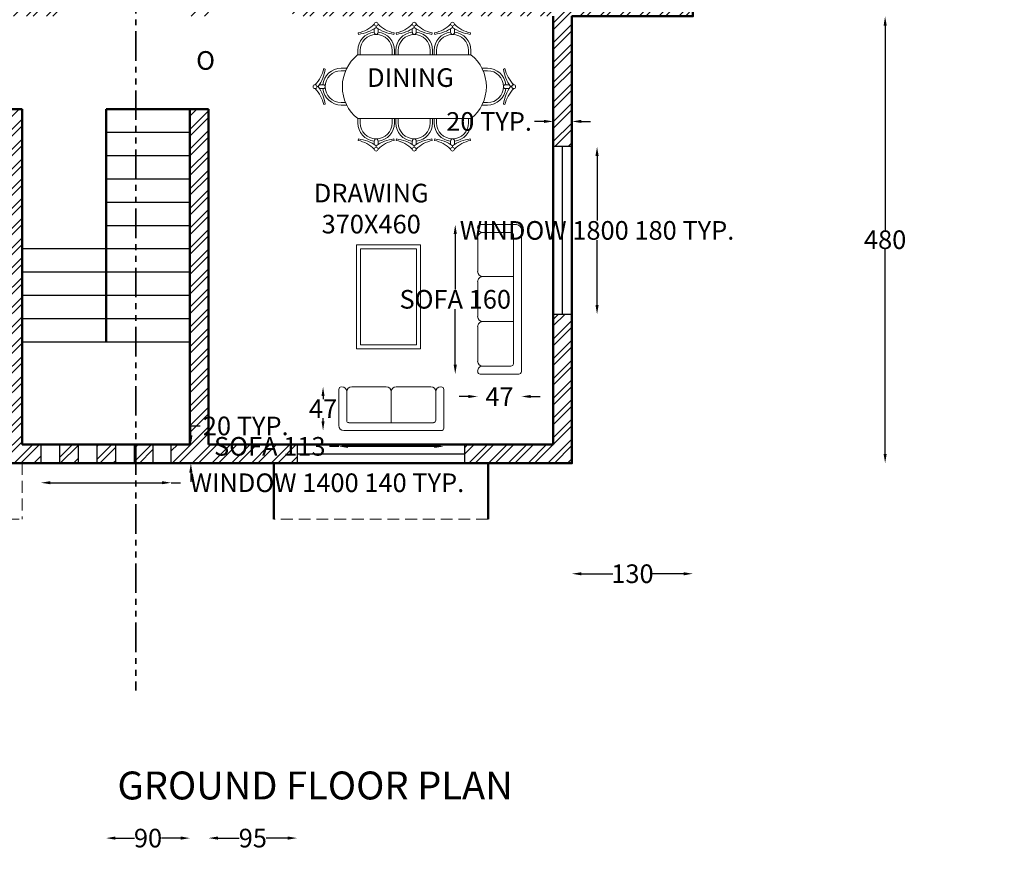
# Model space of a CAD drawing. Units: centimetres. Extents: x 10444 to 13814, y 8288 to 11191.
# Tile 3 of 9: x 11072 to 12129, y 9505 to 10397. Entities that reach past the tile are written whole.
import ezdxf

# ---------------------------------------------------------------- set-up
doc = ezdxf.new("R2010")
doc.units = ezdxf.units.CM
doc.header["$MEASUREMENT"] = 0
doc.linetypes.add('DASHED', pattern=[19.05, 12.7, -6.35])
doc.linetypes.add('PHANTOM', pattern=[63.5, 31.75, -6.35, 6.35, -6.35, 6.35, -6.35])
for name, color, linetype, lineweight in [('A-ANNO-DIMS', 2, 'Continuous', 18), ('A-ANNO-SYMB-SECT', 1, 'PHANTOM', 35), ('A-ANNO-TEXT', 7, 'Continuous', 25), ('A-AREA-IDEN', 3, 'Continuous', 25), ('A-FLOR-STRS', 3, 'Continuous', 25), ('A-FURN', 8, 'Continuous', 18), ('A-GLAZ', 4, 'Continuous', 25), ('A-ROOF-OVHD', 6, 'DASHED', 18), ('A-WALL', 7, 'Continuous', 50), ('A-WALL-PATT', 8, 'Continuous', 13)]:
    doc.layers.add(name, color=color, linetype=linetype, lineweight=lineweight)
doc.styles.get("Standard").update_dxf_attribs({"font": 'arial.ttf'})
doc.dimstyles.get("Standard").update_dxf_attribs({"dimtxt": 20, "dimasz": 10, "dimexe": 0.18, "dimexo": 0.0625, "dimgap": 0.09, "dimtad": 0, "dimtih": 1, "dimtoh": 1, "dimdec": 0, "dimzin": 0, "dimdsep": 46, "dimtxsty": 'Standard', "dimcen": 0.09, "dimse1": 1, "dimse2": 1, "dimadec": 0, "dimazin": 0, "dimtfac": 1, "dimtdec": 0, "dimtofl": 0, "dimtmove": 0, "dimatfit": 3, "dimfxl": 1, "dimtolj": 1, "dimtzin": 0, "dimarcsym": 0})

# ---------------------------------------------------------------- blocks, each defined once
blk = doc.blocks.new('sofa-25')
at = {"color": 0, "linetype": 'ByBlock'}
for p, q in [((-0.03, 0.03), (-0.03, 0.49)), ((0.535, 0.52), (0.124, 0.52)), ((1.07, 0.52), (0.653, 0.52)), ((1.594, 0.52), (1.188, 0.52)), ((1.747, 0.059), (1.747, 0.49)), ((0.065, 0.124), (0.065, 0.461)), ((0.594, 0.094), (0.594, 0.461)), ((1.129, 0.094), (1.129, 0.461)), ((1.653, 0.118), (1.653, 0.461)), ((0, 0), (1.688, 0)), ((0.094, 0.094), (1.629, 0.094))]:
    blk.add_line(p, q, dxfattribs=at)
for centre, radius, start, end in [((0, 0.49), 0.0295, 90, 180), ((0.006, 0.461), 0.0591, 0, 90), ((0.124, 0.461), 0.0591, 90, 180), ((0.535, 0.461), 0.0591, 0, 90), ((0.653, 0.461), 0.0591, 90, 180), ((1.07, 0.461), 0.0591, 0, 90), ((1.188, 0.461), 0.0591, 90, 180), ((1.594, 0.461), 0.0591, 0, 90), ((1.712, 0.461), 0.0591, 90, 180), ((1.718, 0.49), 0.0295, 0, 90), ((0.094, 0.124), 0.0295, 180, 270), ((1.629, 0.118), 0.0236, 270, 0), ((0, 0.03), 0.0295, 180, 270), ((1.688, 0.059), 0.0591, 270, 0)]:
    blk.add_arc(centre, radius, start, end, dxfattribs=at)
blk = doc.blocks.new('sofa-26')
at = {"color": 0, "linetype": 'ByBlock'}
for p, q in [((-0.03, 0.03), (-0.03, 0.49)), ((0.535, 0.52), (0.124, 0.52)), ((1.064, 0.52), (0.653, 0.52)), ((1.218, 0.059), (1.218, 0.49)), ((0.065, 0.124), (0.065, 0.461)), ((0.594, 0.094), (0.594, 0.461)), ((1.123, 0.118), (1.123, 0.461)), ((0, 0), (1.159, 0)), ((0.094, 0.094), (1.1, 0.094))]:
    blk.add_line(p, q, dxfattribs=at)
for centre, radius, start, end in [((0, 0.49), 0.0295, 90, 180), ((0.006, 0.461), 0.0591, 0, 90), ((0.124, 0.461), 0.0591, 90, 180), ((0.535, 0.461), 0.0591, 0, 90), ((0.653, 0.461), 0.0591, 90, 180), ((1.064, 0.461), 0.0591, 0, 90), ((1.182, 0.461), 0.0591, 90, 180), ((1.188, 0.49), 0.0295, 0, 90), ((0.094, 0.124), 0.0295, 180, 270), ((1.1, 0.118), 0.0236, 270, 0), ((0, 0.03), 0.0295, 180, 270), ((1.159, 0.059), 0.0591, 270, 0)]:
    blk.add_arc(centre, radius, start, end, dxfattribs=at)
blk = doc.blocks.new('*D9')
at = {"layer": 'A-ANNO-DIMS', "color": 0, "lineweight": -2, "transparency": 16777216}
for p, q in [((12001, 10390.6), (12001, 10170.9)), ((12001, 9930.6), (12001, 10150.3))]:
    blk.add_line(p, q, dxfattribs=at)
at = {"layer": 'A-ANNO-DIMS', "color": 0, "transparency": 16777216}
for points in [[(11999.4, 10390.6), (12002.7, 10390.6), (12001, 10400.6)], [(11999.4, 9930.6), (12002.7, 9930.6), (12001, 9920.6)]]:
    blk.add_solid(points, dxfattribs=at)
at = {"layer": 'Defpoints', "color": 0, "transparency": 16777216}
for p in [(11664.8, 10400.6), (11664.8, 9920.6), (12001, 9920.6)]:
    blk.add_point(p, dxfattribs=at)
at = {"layer": 'A-ANNO-DIMS', "color": 0, "transparency": 16777216, "insert": (12001, 10160.6), "char_height": 20, "attachment_point": 5}
blk.add_mtext('\\A1;480', dxfattribs=at)
blk = doc.blocks.new('*D14')
at = {"layer": 'A-ANNO-DIMS', "color": 0, "lineweight": -2, "transparency": 16777216}
for p, q in [((11674.8, 9801.9), (11708.6, 9801.9)), ((11784.8, 9801.9), (11751, 9801.9))]:
    blk.add_line(p, q, dxfattribs=at)
at = {"layer": 'A-ANNO-DIMS', "color": 0, "transparency": 16777216}
for points in [[(11674.8, 9803.5), (11674.8, 9800.2), (11664.8, 9801.9)], [(11784.8, 9803.5), (11784.8, 9800.2), (11794.8, 9801.9)]]:
    blk.add_solid(points, dxfattribs=at)
at = {"layer": 'Defpoints', "color": 0, "transparency": 16777216}
for p in [(11664.8, 10400.6), (11794.8, 10400.6), (11664.8, 9801.9)]:
    blk.add_point(p, dxfattribs=at)
at = {"layer": 'A-ANNO-DIMS', "color": 0, "transparency": 16777216, "insert": (11729.8, 9801.9), "char_height": 20, "attachment_point": 5}
blk.add_mtext('\\A1;130', dxfattribs=at)
blk = doc.blocks.new('f')
for p, q in [((11304.7, 9881.5), (11164.7, 9881.5)), ((11164.7, 9881.5), (11164.7, 9861.5)), ((11184.7, 9881.5), (11184.7, 9861.5)), ((11204.7, 9881.5), (11204.7, 9861.5)), ((11224.7, 9881.5), (11224.7, 9861.5)), ((11244.7, 9881.5), (11244.7, 9861.5)), ((11264.7, 9881.5), (11264.7, 9861.5)), ((11284.7, 9881.5), (11284.7, 9861.5)), ((11304.7, 9861.5), (11304.7, 9881.5)), ((11164.7, 9861.5), (11304.7, 9861.5))]:
    blk.add_line(p, q)
blk = doc.blocks.new('WIN-1800')
blk.add_line((0, 10), (180, 10))
blk.add_lwpolyline([(0, 0), (180, 0), (180, 20), (0, 20)], close=True)
blk = doc.blocks.new('*D31')
at = {"layer": 'A-ANNO-DIMS', "color": 0, "lineweight": -2, "transparency": 16777216}
for p, q in [((11691.8, 10250.6), (11691.8, 10181.1)), ((11691.8, 10090.6), (11691.8, 10160.2))]:
    blk.add_line(p, q, dxfattribs=at)
at = {"layer": 'A-ANNO-DIMS', "color": 0, "transparency": 16777216}
for points in [[(11690.1, 10250.6), (11693.5, 10250.6), (11691.8, 10260.6)], [(11690.1, 10090.6), (11693.5, 10090.6), (11691.8, 10080.6)]]:
    blk.add_solid(points, dxfattribs=at)
at = {"layer": 'Defpoints', "color": 0, "transparency": 16777216}
for p in [(11664.8, 10260.6), (11691.8, 10260.6), (11664.8, 10080.6)]:
    blk.add_point(p, dxfattribs=at)
at = {"layer": 'A-ANNO-DIMS', "color": 0, "transparency": 16777216, "insert": (11691.8, 10170.6), "char_height": 20, "attachment_point": 5}
blk.add_mtext('\\A1;WINDOW 1800 180 TYP.', dxfattribs=at)
blk = doc.blocks.new('*D32')
at = {"layer": 'A-ANNO-DIMS', "color": 0, "lineweight": -2, "transparency": 16777216}
for p, q in [((11634.8, 10287.6), (11624.8, 10287.6)), ((11674.8, 10287.6), (11684.8, 10287.6))]:
    blk.add_line(p, q, dxfattribs=at)
at = {"layer": 'A-ANNO-DIMS', "color": 0, "transparency": 16777216}
for points in [[(11634.8, 10289.3), (11634.8, 10286), (11644.8, 10287.6)], [(11674.8, 10289.3), (11674.8, 10286), (11664.8, 10287.6)]]:
    blk.add_solid(points, dxfattribs=at)
at = {"layer": 'Defpoints', "color": 0, "transparency": 16777216}
for p in [(11644.8, 10287.6), (11644.8, 10260.6), (11664.8, 10260.6)]:
    blk.add_point(p, dxfattribs=at)
at = {"layer": 'A-ANNO-DIMS', "color": 0, "transparency": 16777216, "insert": (11575.9, 10287.6), "char_height": 20, "attachment_point": 5}
blk.add_mtext('\\A1;20 TYP.', dxfattribs=at)
blk = doc.blocks.new('*D35')
at = {"layer": 'A-ANNO-DIMS', "color": 0, "lineweight": -2, "transparency": 16777216}
for p, q in [((11104.8, 9899.6), (11224.8, 9899.6)), ((11234.8, 9899.6), (11244.8, 9899.6))]:
    blk.add_line(p, q, dxfattribs=at)
at = {"layer": 'A-ANNO-DIMS', "color": 0, "transparency": 16777216}
for points in [[(11104.8, 9901.3), (11104.8, 9898), (11094.8, 9899.6)], [(11224.8, 9901.3), (11224.8, 9898), (11234.8, 9899.6)]]:
    blk.add_solid(points, dxfattribs=at)
at = {"layer": 'Defpoints', "color": 0, "transparency": 16777216}
for p in [(11094.8, 9920.6), (11234.8, 9920.6), (11234.8, 9899.6)]:
    blk.add_point(p, dxfattribs=at)
at = {"layer": 'A-ANNO-DIMS', "color": 0, "transparency": 16777216, "insert": (11401.9, 9899.6), "char_height": 20, "attachment_point": 5}
blk.add_mtext('\\A1;WINDOW 1400 140 TYP.', dxfattribs=at)
blk = doc.blocks.new('*D36')
at = {"layer": 'A-ANNO-DIMS', "color": 0, "lineweight": -2, "transparency": 16777216}
for p, q in [((11255.8, 9950.6), (11255.8, 9960.6)), ((11255.8, 9960.6), (11265.8, 9960.6)), ((11255.8, 9910.6), (11255.8, 9900.6))]:
    blk.add_line(p, q, dxfattribs=at)
at = {"layer": 'A-ANNO-DIMS', "color": 0, "transparency": 16777216}
for points in [[(11254.1, 9950.6), (11257.5, 9950.6), (11255.8, 9940.6)], [(11254.1, 9910.6), (11257.5, 9910.6), (11255.8, 9920.6)]]:
    blk.add_solid(points, dxfattribs=at)
at = {"layer": 'Defpoints', "color": 0, "transparency": 16777216}
for p in [(11234.8, 9940.6), (11255.8, 9940.6), (11234.8, 9920.6)]:
    blk.add_point(p, dxfattribs=at)
at = {"layer": 'A-ANNO-DIMS', "color": 0, "transparency": 16777216, "insert": (11314.7, 9960.6), "char_height": 20, "attachment_point": 5}
blk.add_mtext('\\A1;20 TYP.', dxfattribs=at)
blk = doc.blocks.new('*D45')
at = {"layer": 'A-ANNO-DIMS', "color": 0, "lineweight": -2, "transparency": 16777216}
for p, q in [((11539.6, 10166.8), (11539.6, 10107)), ((11539.6, 10026.3), (11539.6, 10086.1))]:
    blk.add_line(p, q, dxfattribs=at)
at = {"layer": 'A-ANNO-DIMS', "color": 0, "transparency": 16777216}
for points in [[(11537.9, 10166.8), (11541.3, 10166.8), (11539.6, 10176.8)], [(11537.9, 10026.3), (11541.3, 10026.3), (11539.6, 10016.3)]]:
    blk.add_solid(points, dxfattribs=at)
at = {"layer": 'Defpoints', "color": 0, "transparency": 16777216}
for p in [(11539.6, 10176.8), (11563.7, 10176.8), (11563.7, 10016.3)]:
    blk.add_point(p, dxfattribs=at)
at = {"layer": 'A-ANNO-DIMS', "color": 0, "transparency": 16777216, "insert": (11539.6, 10096.6), "char_height": 20, "attachment_point": 5}
blk.add_mtext('\\A1;SOFA 160', dxfattribs=at)
blk = doc.blocks.new('*D46')
at = {"layer": 'A-ANNO-DIMS', "color": 0, "lineweight": -2, "transparency": 16777216}
for p, q in [((11553.7, 9992.2), (11543.7, 9992.2)), ((11620.6, 9992.2), (11630.6, 9992.2))]:
    blk.add_line(p, q, dxfattribs=at)
at = {"layer": 'A-ANNO-DIMS', "color": 0, "transparency": 16777216}
for points in [[(11553.7, 9993.9), (11553.7, 9990.6), (11563.7, 9992.2)], [(11620.6, 9993.9), (11620.6, 9990.6), (11610.6, 9992.2)]]:
    blk.add_solid(points, dxfattribs=at)
at = {"layer": 'Defpoints', "color": 0, "transparency": 16777216}
for p in [(11563.7, 10016.3), (11610.6, 10016.3), (11563.7, 9992.2)]:
    blk.add_point(p, dxfattribs=at)
at = {"layer": 'A-ANNO-DIMS', "color": 0, "transparency": 16777216, "insert": (11587.1, 9992.2), "char_height": 20, "attachment_point": 5}
blk.add_mtext('\\A1;47', dxfattribs=at)
blk = doc.blocks.new('*D47')
at = {"layer": 'A-ANNO-DIMS', "color": 0, "lineweight": -2, "transparency": 16777216}
for p, q in [((11414.6, 9938.7), (11404.6, 9938.7)), ((11517.2, 9938.7), (11424.6, 9938.7))]:
    blk.add_line(p, q, dxfattribs=at)
at = {"layer": 'A-ANNO-DIMS', "color": 0, "transparency": 16777216}
for points in [[(11424.6, 9940.4), (11424.6, 9937), (11414.6, 9938.7)], [(11517.2, 9940.4), (11517.2, 9937), (11527.2, 9938.7)]]:
    blk.add_solid(points, dxfattribs=at)
at = {"layer": 'Defpoints', "color": 0, "transparency": 16777216}
for p in [(11414.6, 9955.6), (11527.2, 9955.6), (11414.6, 9938.7)]:
    blk.add_point(p, dxfattribs=at)
at = {"layer": 'A-ANNO-DIMS', "color": 0, "transparency": 16777216, "insert": (11340.5, 9938.7), "char_height": 20, "attachment_point": 5}
blk.add_mtext('\\A1;SOFA 113', dxfattribs=at)
blk = doc.blocks.new('*D48')
at = {"layer": 'A-ANNO-DIMS', "color": 0, "lineweight": -2, "transparency": 16777216}
for p, q in [((11397.7, 9992.6), (11397.7, 9989.2)), ((11397.7, 9965.6), (11397.7, 9969))]:
    blk.add_line(p, q, dxfattribs=at)
at = {"layer": 'A-ANNO-DIMS', "color": 0, "transparency": 16777216}
for points in [[(11396, 9992.6), (11399.3, 9992.6), (11397.7, 10002.6)], [(11396, 9965.6), (11399.3, 9965.6), (11397.7, 9955.6)]]:
    blk.add_solid(points, dxfattribs=at)
at = {"layer": 'Defpoints', "color": 0, "transparency": 16777216}
for p in [(11397.7, 10002.6), (11414.6, 10002.6), (11414.6, 9955.6)]:
    blk.add_point(p, dxfattribs=at)
at = {"layer": 'A-ANNO-DIMS', "color": 0, "transparency": 16777216, "insert": (11397.7, 9979.1), "char_height": 20, "attachment_point": 5}
blk.add_mtext('\\A1;47', dxfattribs=at)
blk = doc.blocks.new('*D76')
at = {"layer": 'A-ANNO-DIMS', "color": 0, "lineweight": -2, "transparency": 16777216}
for p, q in [((10466.3, 10390.6), (10466.3, 10360.9)), ((10466.3, 10310.6), (10466.3, 10340.3))]:
    blk.add_line(p, q, dxfattribs=at)
at = {"layer": 'A-ANNO-DIMS', "color": 0, "transparency": 16777216}
for points in [[(10464.6, 10390.6), (10468, 10390.6), (10466.3, 10400.6)], [(10464.6, 10310.6), (10468, 10310.6), (10466.3, 10300.6)]]:
    blk.add_solid(points, dxfattribs=at)
at = {"layer": 'Defpoints', "color": 0, "transparency": 16777216}
for p in [(10466.3, 10400.6), (11114.8, 10400.6), (11054.8, 10300.6)]:
    blk.add_point(p, dxfattribs=at)
at = {"layer": 'A-ANNO-DIMS', "color": 0, "transparency": 16777216, "insert": (10466.3, 10350.6), "char_height": 20, "attachment_point": 5}
blk.add_mtext('\\A1;100', dxfattribs=at)
blk = doc.blocks.new('*D81')
at = {"layer": 'A-ANNO-DIMS', "color": 0, "lineweight": -2, "transparency": 16777216}
for p, q in [((10466.3, 10070.6), (10466.3, 10010.9)), ((10466.3, 9930.6), (10466.3, 9990.3))]:
    blk.add_line(p, q, dxfattribs=at)
at = {"layer": 'A-ANNO-DIMS', "color": 0, "transparency": 16777216}
for points in [[(10464.6, 10070.6), (10468, 10070.6), (10466.3, 10080.6)], [(10464.6, 9930.6), (10468, 9930.6), (10466.3, 9920.6)]]:
    blk.add_solid(points, dxfattribs=at)
at = {"layer": 'Defpoints', "color": 0, "transparency": 16777216}
for p in [(10466.3, 10080.6), (11664.8, 10080.6), (11664.8, 9920.6)]:
    blk.add_point(p, dxfattribs=at)
at = {"layer": 'A-ANNO-DIMS', "color": 0, "transparency": 16777216, "insert": (10466.3, 10000.6), "char_height": 20, "attachment_point": 5}
blk.add_mtext('\\A1;160', dxfattribs=at)
blk = doc.blocks.new('*D82')
at = {"layer": 'A-ANNO-DIMS', "color": 0, "lineweight": -2, "transparency": 16777216}
for p, q in [((11284.8, 9518), (11307.8, 9518)), ((11359.8, 9518), (11336.8, 9518))]:
    blk.add_line(p, q, dxfattribs=at)
at = {"layer": 'A-ANNO-DIMS', "color": 0, "transparency": 16777216}
for points in [[(11284.8, 9519.7), (11284.8, 9516.3), (11274.8, 9518)], [(11359.8, 9519.7), (11359.8, 9516.3), (11369.8, 9518)]]:
    blk.add_solid(points, dxfattribs=at)
at = {"layer": 'Defpoints', "color": 0, "transparency": 16777216}
for p in [(11274.8, 9940.6), (11369.8, 9920.6), (11369.8, 9518)]:
    blk.add_point(p, dxfattribs=at)
at = {"layer": 'A-ANNO-DIMS', "color": 0, "transparency": 16777216, "insert": (11322.3, 9518), "char_height": 20, "attachment_point": 5}
blk.add_mtext('\\A1;95', dxfattribs=at)
blk = doc.blocks.new('*D84')
at = {"layer": 'A-ANNO-DIMS', "color": 0, "lineweight": -2, "transparency": 16777216}
for p, q in [((11174.8, 9518), (11195.4, 9518)), ((11244.8, 9518), (11224.2, 9518))]:
    blk.add_line(p, q, dxfattribs=at)
at = {"layer": 'A-ANNO-DIMS', "color": 0, "transparency": 16777216}
for points in [[(11174.8, 9519.7), (11174.8, 9516.3), (11164.8, 9518)], [(11244.8, 9519.7), (11244.8, 9516.3), (11254.8, 9518)]]:
    blk.add_solid(points, dxfattribs=at)
at = {"layer": 'Defpoints', "color": 0, "transparency": 16777216}
for p in [(11164.8, 10300.6), (11254.8, 10300.6), (11254.8, 9518)]:
    blk.add_point(p, dxfattribs=at)
at = {"layer": 'A-ANNO-DIMS', "color": 0, "transparency": 16777216, "insert": (11209.8, 9518), "char_height": 20, "attachment_point": 5}
blk.add_mtext('\\A1;90', dxfattribs=at)
blk = doc.blocks.new('*D85')
at = {"layer": 'A-ANNO-DIMS', "color": 0, "lineweight": -2, "transparency": 16777216}
for p, q in [((10466.3, 10285.6), (10466.3, 10295.6)), ((10466.3, 10240.6), (10466.3, 10230.6))]:
    blk.add_line(p, q, dxfattribs=at)
at = {"layer": 'A-ANNO-DIMS', "color": 0, "transparency": 16777216}
for points in [[(10464.6, 10285.6), (10468, 10285.6), (10466.3, 10275.6)], [(10464.6, 10240.6), (10468, 10240.6), (10466.3, 10250.6)]]:
    blk.add_solid(points, dxfattribs=at)
at = {"layer": 'Defpoints', "color": 0, "transparency": 16777216}
for p in [(11164.8, 10275.6), (10466.3, 10250.6), (11164.8, 10250.6)]:
    blk.add_point(p, dxfattribs=at)
at = {"layer": 'A-ANNO-DIMS', "color": 0, "transparency": 16777216, "insert": (10466.3, 10263.1), "char_height": 20, "attachment_point": 5}
blk.add_mtext('\\A1;25', dxfattribs=at)

msp = doc.modelspace()

# ---------------------------------------------------------------- hatches: boundary and pattern name
at = {"layer": 'A-WALL-PATT'}
h = msp.add_hatch(dxfattribs=at)
h.set_pattern_fill('ANSI32', color=256, scale=40)
h.paths.add_polyline_path([(10809.7881, 10800.6336), (10684.7881, 10800.6336), (10684.7881, 10690.6336), (10704.7881, 10690.6336), (10704.7881, 10726.41), (10704.7881, 10780.6336), (10809.7881, 10780.6336)])
h.paths.add_polyline_path([(11154.7881, 10800.6336), (10989.7881, 10800.6336), (10989.7881, 10780.6336), (11114.7881, 10780.6336), (11154.7881, 10780.6336)])
h.paths.add_polyline_path([(11354.7881, 10800.6336), (11214.7881, 10800.6336), (11214.7881, 10780.6336), (11254.7881, 10780.6336), (11254.7881, 10582.9925, -0.004993085), (11254.7881, 10581.0383), (11254.7881, 10571.0719, -0.269473124), (11256.5873, 10571.9821), (11256.5873, 10568.3227), (11256.5873, 10564.4272, -0.269473124), (11254.7881, 10565.3375), (11254.7881, 10530.6336), (11196.6819, 10530.6336), (11196.6819, 10510.6336), (11254.7881, 10510.6336), (11254.7881, 10400.6336), (11274.7881, 10400.6336), (11274.7881, 10420.6336), (11274.7881, 10780.6336), (11354.7881, 10780.6336)])
h.paths.add_polyline_path([(10704.7881, 10510.6336), (10684.7881, 10510.6336), (10684.7881, 10400.6336), (10734.7881, 10400.6336), (10734.7881, 10340.6336), (10754.7881, 10340.6336), (10754.7881, 10400.6336), (11114.7881, 10400.6336), (11114.7881, 10420.6336), (10704.7881, 10420.6336)])
h.paths.add_polyline_path([(11794.7881, 10420.6336), (11364.7881, 10420.6336), (11364.7881, 10400.6336), (11644.7881, 10400.6336), (11644.7881, 10260.6336), (11664.7881, 10260.6336), (11664.7881, 10400.6336), (11794.7881, 10400.6336)])
h.paths.add_polyline_path([(11594.7881, 10670.6336), (11594.7881, 10708.9482, -0.268280405), (11592.9938, 10708.0455), (11592.9938, 10711.9409), (11592.9938, 10715.6003, -0.268280405), (11594.7881, 10714.6976), (11594.7881, 10780.6336), (11654.7881, 10780.6336), (11654.7881, 10800.6336), (11494.7881, 10800.6336), (11494.7881, 10780.6336), (11574.7881, 10780.6336), (11574.7881, 10510.6336), (11594.7881, 10510.6336)])
h.paths.add_polyline_path([(11794.7881, 10800.6336), (11714.7881, 10800.6336), (11714.7881, 10780.6336), (11774.7881, 10780.6336), (11774.7881, 10750.6336), (11794.7881, 10750.6336)])
h.paths.add_polyline_path([(11794.7881, 10670.6336), (11674.7881, 10670.6336), (11674.7881, 10650.6336), (11794.7881, 10650.6336)])
h.paths.add_polyline_path([(11664.7881, 10080.6336), (11644.7881, 10080.6336), (11644.7881, 9940.6336), (11549.7881, 9940.6336), (11549.7881, 9920.6336), (11664.7881, 9920.6336)])
h.paths.add_polyline_path([(11369.7881, 9940.6336), (11274.7881, 9940.6336), (11274.7881, 10300.6336), (11254.7881, 10300.6336), (11254.7881, 9940.6336), (11234.7881, 9940.6336), (11234.7881, 9920.6336), (11369.7881, 9920.6336)])
h.paths.add_polyline_path([(11094.7881, 9940.6336), (11074.7881, 9940.6336), (11074.7881, 10300.6336), (11054.7881, 10300.6336), (11054.7881, 10080.6336), (11054.7881, 9920.6336), (11094.7881, 9920.6336)])
h.paths.add_polyline_path([(11134.7881, 9940.6336), (11114.7881, 9940.6336), (11114.7881, 9920.6336), (11134.7881, 9920.6336)])
h.paths.add_polyline_path([(11174.7881, 9940.6336), (11154.7881, 9940.6336), (11154.7881, 9920.6336), (11174.7881, 9920.6336)])
h.paths.add_polyline_path([(11214.7881, 9940.6336), (11196.6819, 9940.6336), (11196.6819, 9920.6336), (11214.7881, 9920.6336)])
h.paths.add_polyline_path([(10954.7881, 10100.6336), (10874.7881, 10100.6336), (10874.7881, 10080.6336), (10954.7881, 10080.6336)])
h.paths.add_polyline_path([(10814.7881, 10100.6336), (10754.7881, 10100.6336), (10754.7881, 10160.6336), (10734.7881, 10160.6336), (10734.7881, 10080.6336), (10814.7881, 10080.6336)])
h.paths.add_polyline_path([(11255.1494, 10331.8339), (11286.882, 10331.8339), (11286.882, 10373.0481), (11255.1494, 10373.0481)], flags=9)
h.paths.add_polyline_path([(11607.8445, 10630.7128), (11653.5607, 10630.7128), (11653.5607, 10671.927), (11607.8445, 10671.927)], flags=25)
h.paths.add_polyline_path([(11746.8445, 10447.0791), (11792.5607, 10447.0791), (11792.5607, 10488.2933), (11746.8445, 10488.2933)], flags=9)
h.paths.add_polyline_path([(11296.8445, 10388.5791), (11342.5607, 10388.5791), (11342.5607, 10429.7933), (11296.8445, 10429.7933)], flags=9)
h.paths.add_polyline_path([(11376.6416, 10156.0222), (11521.6757, 10156.0222), (11521.6757, 10230.6515), (11376.6416, 10230.6515)], flags=9)
h.paths.add_polyline_path([(11437.3982, 10313.4478), (11545.1881, 10313.4478), (11545.1881, 10354.662), (11437.3982, 10354.662)], flags=25)
h.paths.add_polyline_path([(11655.4027, 10682.0329), (11777.2718, 10682.0329), (11777.2718, 10756.6623), (11655.4027, 10756.6623)], flags=9)
h.paths.add_polyline_path([(11636.2626, 10500.0811), (11758.1316, 10500.0811), (11758.1316, 10574.7105), (11636.2626, 10574.7105)], flags=9)
h.paths.add_polyline_path([(11336.6251, 10562.3234), (11469.2581, 10562.3234), (11469.2581, 10636.9528), (11336.6251, 10636.9528)], flags=9)
h = msp.add_hatch(dxfattribs=at)
h.set_pattern_fill('ANSI32', color=256, scale=40)
h.paths.add_polyline_path([(12933.1062, 10800.6336), (12768.1062, 10800.6336), (12768.1062, 10780.6336), (12933.1062, 10780.6336)])
h.paths.add_polyline_path([(12588.1062, 10800.6336), (12463.1062, 10800.6336), (12463.1062, 10780.6336), (12588.1062, 10780.6336)])
h.paths.add_polyline_path([(12483.1062, 10726.41), (12483.1062, 10780.6336), (12463.1062, 10780.6336), (12463.1062, 10690.6336), (12483.1062, 10690.6336)])
h.paths.add_polyline_path([(12483.1062, 10510.6336), (12463.1062, 10510.6336), (12463.1062, 10400.6336), (12510.094, 10400.6336), (12529.0899, 10420.6336), (12483.1062, 10420.6336)])
h.paths.add_polyline_path([(12699.6814, 10420.6336), (12529.0899, 10420.6336), (12510.094, 10400.6336), (12513.1062, 10400.6336), (12513.1062, 10340.6336), (12533.1062, 10340.6336), (12533.1062, 10400.6336), (12699.64, 10400.6336)])
h.paths.add_polyline_path([(12893.1062, 10420.6336), (12699.6814, 10420.6336), (12699.64, 10400.6336), (12893.1062, 10400.6336)])
h.paths.add_polyline_path([(13129.7438, 10800.6336), (12993.1062, 10800.6336), (12993.1062, 10780.6336), (13033.1062, 10780.6336), (13033.1062, 10600.6336), (13053.1062, 10600.6336), (13053.1062, 10780.6336), (13129.7438, 10780.6336)])
h.paths.add_polyline_path([(13433.1062, 10800.6336), (13309.7438, 10800.6336), (13309.7438, 10780.6336), (13345.5201, 10780.6336), (13353.1062, 10780.6336), (13353.1062, 10600.6336), (13373.1062, 10600.6336), (13373.1062, 10780.6336), (13433.1062, 10780.6336)])
h.paths.add_polyline_path([(13573.1062, 10800.6336), (13493.1062, 10800.6336), (13493.1062, 10780.6336), (13553.1062, 10780.6336), (13553.1062, 10600.6336), (13573.1062, 10600.6336)])
h.paths.add_polyline_path([(13573.1062, 10600.6336), (13553.1062, 10600.6336), (13553.1062, 10420.6336), (13053.1062, 10420.6336), (13053.1062, 10400.6336), (13573.1062, 10400.6336)])
h.paths.add_polyline_path([(13053.1062, 10300.6336), (13033.1062, 10300.6336), (13033.1062, 9940.6336), (13013.1062, 9940.6336), (13013.1062, 9920.6336), (13053.1062, 9920.6336)])
h.paths.add_polyline_path([(12993.1062, 9940.6336), (12975, 9940.6336), (12975, 9920.6336), (12993.1062, 9920.6336)])
h.paths.add_polyline_path([(12953.1062, 9940.6336), (12933.1062, 9940.6336), (12933.1062, 9920.6336), (12953.1062, 9920.6336)])
h.paths.add_polyline_path([(12913.1062, 9940.6336), (12893.1062, 9940.6336), (12893.1062, 9920.6336), (12913.1062, 9920.6336)])
h.paths.add_polyline_path([(12873.1062, 9940.6336), (12853.1062, 9940.6336), (12853.1062, 10300.6336), (12833.1062, 10300.6336), (12833.1062, 9920.6336), (12873.1062, 9920.6336)])
h.paths.add_polyline_path([(12733.1062, 10100.6336), (12699.0201, 10100.6336), (12698.9788, 10080.6336), (12733.1062, 10080.6336)])
h.paths.add_polyline_path([(12699.0201, 10100.6336), (12653.1062, 10100.6336), (12653.1062, 10080.6336), (12698.9788, 10080.6336)])
h.paths.add_polyline_path([(12593.1062, 10100.6336), (12533.1062, 10100.6336), (12533.1062, 10160.6336), (12513.1062, 10160.6336), (12513.1062, 10080.6336), (12593.1062, 10080.6336)])
h.paths.add_polyline_path([(13053.1062, 10600.6336), (13033.1062, 10600.6336), (13033.1062, 10576.2537, -0.004993085), (13033.1062, 10574.2995), (13033.1062, 10564.3331, -0.269473124), (13034.9053, 10565.2433), (13034.9053, 10561.5839), (13034.9053, 10557.6884, -0.269473124), (13033.1062, 10558.5987), (13033.1062, 10530.6336), (12975, 10530.6336), (12975, 10510.6336), (13053.1062, 10510.6336)])
h.paths.add_polyline_path([(12975, 10530.6336), (12893.1062, 10530.6336), (12893.1062, 10600.6336), (12873.1062, 10600.6336), (12873.1062, 10510.6336), (12975, 10510.6336)])
h.paths.add_polyline_path([(12893.1062, 10700.6336), (12873.1062, 10700.6336), (12873.1062, 10600.6336), (12893.1062, 10600.6336)])
h.paths.add_polyline_path([(13373.1062, 10600.6336), (13353.1062, 10600.6336), (13353.1062, 10507.9506), (13373.1062, 10507.9506)], flags=17)
h.paths.add_polyline_path([(13553.1062, 10620.6336), (13453.1062, 10620.6336), (13453.1062, 10600.6336), (13553.1062, 10600.6336)])
h.paths.add_polyline_path([(11114.7881, 10700.6336), (11094.7881, 10700.6336), (11094.7881, 10510.6336), (11196.6819, 10510.6336), (11196.6819, 10530.6336), (11114.7881, 10530.6336)])

# ---------------------------------------------------------------- linework, layer by layer
at = {"layer": 'A-ANNO-SYMB-SECT'}
msp.add_line((11196.6819, 11019.5), (11196.6819, 9676.5), dxfattribs=at)
at = {"layer": 'A-FLOR-STRS'}
for p, q in [((11254.7881, 10275.6336), (11164.7881, 10275.6336)), ((11254.7881, 10250.6336), (11164.7881, 10250.6336)), ((11254.7881, 10225.6336), (11164.7881, 10225.6336)), ((11254.7881, 10200.6336), (11164.7881, 10200.6336)), ((11254.7881, 10175.6336), (11164.7881, 10175.6336)), ((11254.7881, 10150.6336), (11074.7881, 10150.6336)), ((11254.7881, 10125.6336), (11074.7881, 10125.6336)), ((11254.7881, 10100.6336), (11074.7881, 10100.6336)), ((11254.7881, 10075.6336), (11074.7881, 10075.6336)), ((11254.7881, 10050.6336), (11074.7881, 10050.6336))]:
    msp.add_line(p, q, dxfattribs=at)
at = {"layer": 'A-FURN'}
for p, q in [((11454.7059, 10394.2028), (11454.7059, 10394.1203)), ((11454.7059, 10389.985), (11454.7059, 10388.5443)), ((11495.57, 10394.2028), (11495.57, 10394.1203)), ((11495.57, 10389.985), (11495.57, 10388.5443)), ((11536.6788, 10394.2028), (11536.6788, 10394.1203)), ((11536.6788, 10389.985), (11536.6788, 10388.5443)), ((11435.3656, 10382.6492), (11435.8034, 10381.127)), ((11452.6383, 10387.1669), (11452.6383, 10383.5662)), ((11456.7736, 10387.1669), (11456.7736, 10383.5662)), ((11474.0462, 10382.6492), (11473.6084, 10381.127)), ((11476.2297, 10382.6492), (11476.6675, 10381.127)), ((11493.5024, 10387.1669), (11493.5024, 10383.5662)), ((11497.6377, 10387.1669), (11497.6377, 10383.5662)), ((11514.9103, 10382.6492), (11514.4725, 10381.127)), ((11517.3385, 10382.6492), (11517.7764, 10381.127)), ((11534.6112, 10387.1669), (11534.6112, 10383.5662)), ((11538.7465, 10387.1669), (11538.7465, 10383.5662)), ((11556.0192, 10382.6492), (11555.5813, 10381.127)), ((11434.9658, 10363.9346), (11434.9658, 10359.3028)), ((11434.9658, 10363.9346), (11434.9658, 10359.3028)), ((11434.9658, 10359.3028), (11556.419, 10359.3028)), ((11437.5978, 10363.9346), (11437.5978, 10359.2345)), ((11471.814, 10363.9346), (11471.814, 10359.2345)), ((11474.446, 10363.9346), (11474.446, 10359.3028)), ((11475.8299, 10363.9346), (11475.8299, 10359.3028)), ((11475.8299, 10363.9346), (11475.8299, 10359.3028)), ((11478.4619, 10363.9346), (11478.4619, 10359.2345)), ((11512.6781, 10363.9346), (11512.6781, 10359.2345)), ((11515.3101, 10363.9346), (11515.3101, 10359.3028)), ((11516.9387, 10363.9346), (11516.9387, 10359.3028)), ((11516.9387, 10363.9346), (11516.9387, 10359.3028)), ((11519.5708, 10363.9346), (11519.5708, 10359.2345)), ((11553.7869, 10363.9346), (11553.7869, 10359.2345)), ((11556.419, 10363.9346), (11556.419, 10359.3028)), ((11398.4623, 10344.3099), (11399.9845, 10343.8721)), ((11417.1769, 10344.7097), (11423.096, 10344.7097)), ((11417.1769, 10342.0777), (11421.8771, 10342.0777)), ((11574.2079, 10344.7097), (11568.2888, 10344.7097)), ((11574.2079, 10344.7097), (11568.2888, 10344.7097)), ((11574.2079, 10342.0777), (11569.5077, 10342.0777)), ((11592.9224, 10344.3099), (11591.4003, 10343.8721)), ((11393.9447, 10327.0373), (11397.5454, 10327.0373)), ((11597.4401, 10327.0373), (11593.8394, 10327.0373)), ((11386.9088, 10324.9696), (11386.9913, 10324.9696)), ((11391.1266, 10324.9696), (11392.5673, 10324.9696)), ((11393.9447, 10322.902), (11397.5454, 10322.902)), ((11597.4401, 10322.902), (11593.8394, 10322.902)), ((11600.2582, 10324.9696), (11598.8175, 10324.9696)), ((11604.476, 10324.9696), (11604.3935, 10324.9696)), ((11398.4623, 10305.6293), (11399.9845, 10306.0671)), ((11417.1769, 10307.8615), (11421.8771, 10307.8615)), ((11417.1769, 10305.2295), (11423.096, 10305.2295)), ((11574.2079, 10305.2295), (11568.2888, 10305.2295)), ((11574.2079, 10307.8615), (11569.5077, 10307.8615)), ((11592.9224, 10305.6293), (11591.4003, 10306.0671)), ((11434.9658, 10290.6365), (11556.419, 10290.6365)), ((11434.9658, 10286.0046), (11434.9658, 10290.6365)), ((11434.9658, 10286.0046), (11434.9658, 10290.6365)), ((11437.5978, 10286.0046), (11437.5978, 10290.7048)), ((11471.814, 10286.0046), (11471.814, 10290.7048)), ((11474.446, 10286.0046), (11474.446, 10290.6365)), ((11475.8299, 10286.0046), (11475.8299, 10290.6365)), ((11475.8299, 10286.0046), (11475.8299, 10290.6365)), ((11478.4619, 10286.0046), (11478.4619, 10290.7048)), ((11512.6781, 10286.0046), (11512.6781, 10290.7048)), ((11515.3101, 10286.0046), (11515.3101, 10290.6365)), ((11516.9387, 10286.0046), (11516.9387, 10290.6365)), ((11516.9387, 10286.0046), (11516.9387, 10290.6365)), ((11519.5708, 10286.0046), (11519.5708, 10290.7048)), ((11553.7869, 10286.0046), (11553.7869, 10290.7048)), ((11556.419, 10286.0046), (11556.419, 10290.6365)), ((11435.3656, 10267.29), (11435.8034, 10268.8122)), ((11452.6383, 10262.7724), (11452.6383, 10266.3731)), ((11456.7736, 10262.7724), (11456.7736, 10266.3731)), ((11474.0462, 10267.29), (11473.6084, 10268.8122)), ((11476.2297, 10267.29), (11476.6675, 10268.8122)), ((11493.5024, 10262.7724), (11493.5024, 10266.3731)), ((11497.6377, 10262.7724), (11497.6377, 10266.3731)), ((11514.9103, 10267.29), (11514.4725, 10268.8122)), ((11517.3385, 10267.29), (11517.7764, 10268.8122)), ((11534.6112, 10262.7724), (11534.6112, 10266.3731)), ((11538.7465, 10262.7724), (11538.7465, 10266.3731)), ((11556.0192, 10267.29), (11555.5813, 10268.8122)), ((11454.7059, 10259.9542), (11454.7059, 10261.395)), ((11454.7059, 10255.7364), (11454.7059, 10255.8189)), ((11495.57, 10259.9542), (11495.57, 10261.395)), ((11495.57, 10255.7364), (11495.57, 10255.8189)), ((11536.6788, 10259.9542), (11536.6788, 10261.395)), ((11536.6788, 10255.7364), (11536.6788, 10255.8189))]:
    msp.add_line(p, q, dxfattribs=at)
msp.add_lwpolyline([(11475.8299, 10359.3028), (11515.3101, 10359.3028)], dxfattribs=at)
for points in [[(11433.4457, 10043.4895), (11502.112, 10043.4895), (11502.112, 10155.0723), (11433.4457, 10155.0723)], [(11437.7374, 10047.7811), (11497.8204, 10047.7811), (11497.8204, 10150.7806), (11437.7374, 10150.7806)]]:
    msp.add_lwpolyline(points, close=True, dxfattribs=at)
for centre in [(11454.7059, 10392.0526), (11495.57, 10392.0526), (11536.6788, 10392.0526), (11389.0589, 10324.9696), (11602.3259, 10324.9696), (11454.7059, 10257.8866), (11495.57, 10257.8866), (11536.6788, 10257.8866)]:
    msp.add_circle(centre, 2.0676, dxfattribs=at)
for centre, radius, start, end in [((11427.7949, 10417.1209), 35.2932, 282.3867633, 314.7418927), ((11481.617, 10417.1209), 35.2932, 225.2581073, 257.6132367), ((11468.659, 10417.1209), 35.2932, 282.3867633, 314.7418927), ((11522.481, 10417.1209), 35.2932, 225.2581073, 257.6132367), ((11509.7678, 10417.1209), 35.2932, 282.3867633, 314.7418927), ((11563.5899, 10417.1209), 35.2932, 225.2581073, 257.6132367), ((11454.7059, 10363.9346), 19.7401, 96.0123935, 180), ((11430.3067, 10422.9301), 42.1629, 277.4909908, 305.3585107), ((11454.7059, 10363.9346), 17.1081, 0, 180), ((11454.7059, 10383.1104), 2.0676, 167.111565, 12.888435), ((11479.1052, 10422.9301), 42.1629, 234.6414893, 262.5090092), ((11454.7059, 10363.9346), 19.7401, 0, 83.9876065), ((11495.57, 10363.9346), 19.7401, 96.0123935, 180), ((11471.1707, 10422.9301), 42.1629, 277.4909908, 305.3585107), ((11495.57, 10363.9346), 17.1081, 0, 180), ((11495.57, 10383.1104), 2.0676, 167.111565, 12.888435), ((11519.9693, 10422.9301), 42.1629, 234.6414893, 262.5090092), ((11495.57, 10363.9346), 19.7401, 0, 83.9876065), ((11536.6788, 10363.9346), 19.7401, 96.0123935, 180), ((11512.2796, 10422.9301), 42.1629, 277.4909908, 305.3585107), ((11536.6788, 10363.9346), 17.1081, 0, 180), ((11536.6788, 10383.1104), 2.0676, 167.111565, 12.888435), ((11561.0781, 10422.9301), 42.1629, 234.6414893, 262.5090092), ((11536.6788, 10363.9346), 19.7401, 0, 83.9876065), ((11462.2704, 10324.9696), 43.8669, 128.3136983, 231.5053855), ((11529.1144, 10324.9696), 43.8669, 308.4946145, 51.5053855), ((11363.9907, 10351.8807), 35.2932, 315.2581073, 347.6132367), ((11358.1815, 10349.3689), 42.1629, 324.6414893, 352.5090092), ((11417.1769, 10324.9696), 19.7401, 90, 173.9876065), ((11417.1769, 10324.9696), 17.1081, 90, 270), ((11574.2079, 10324.9696), 19.7401, 6.0123935, 90), ((11574.2079, 10324.9696), 17.1081, 270, 90), ((11633.2033, 10349.3689), 42.1629, 187.4909908, 215.3585107), ((11627.3941, 10351.8807), 35.2932, 192.3867633, 224.7418927), ((11398.0012, 10324.9696), 2.0676, 257.111565, 102.888435), ((11593.3836, 10324.9696), 2.0676, 77.111565, 282.888435), ((11363.9907, 10298.0586), 35.2932, 12.3867633, 44.7418927), ((11358.1815, 10300.5703), 42.1629, 7.4909908, 35.3585107), ((11417.1769, 10324.9696), 19.7401, 186.0123935, 270), ((11574.2079, 10324.9696), 19.7401, 270, 353.9876065), ((11633.2033, 10300.5703), 42.1629, 144.6414893, 172.5090092), ((11627.3941, 10298.0586), 35.2932, 135.2581073, 167.6132367), ((11454.7059, 10286.0046), 19.7401, 180, 263.9876065), ((11454.7059, 10286.0046), 17.1081, 180, 0), ((11454.7059, 10286.0046), 19.7401, 276.0123935, 0), ((11495.57, 10286.0046), 19.7401, 180, 263.9876065), ((11495.57, 10286.0046), 17.1081, 180, 0), ((11495.57, 10286.0046), 19.7401, 276.0123935, 0), ((11536.6788, 10286.0046), 19.7401, 180, 263.9876065), ((11536.6788, 10286.0046), 17.1081, 180, 0), ((11536.6788, 10286.0046), 19.7401, 276.0123935, 0), ((11427.7949, 10232.8184), 35.2932, 45.2581073, 77.6132367), ((11430.3067, 10227.0091), 42.1629, 54.6414893, 82.5090092), ((11454.7059, 10266.8289), 2.0676, 347.111565, 192.888435), ((11479.1052, 10227.0091), 42.1629, 97.4909908, 125.3585107), ((11481.617, 10232.8184), 35.2932, 102.3867633, 134.7418927), ((11468.659, 10232.8184), 35.2932, 45.2581073, 77.6132367), ((11471.1707, 10227.0091), 42.1629, 54.6414893, 82.5090092), ((11495.57, 10266.8289), 2.0676, 347.111565, 192.888435), ((11519.9693, 10227.0091), 42.1629, 97.4909908, 125.3585107), ((11522.481, 10232.8184), 35.2932, 102.3867633, 134.7418927), ((11509.7678, 10232.8184), 35.2932, 45.2581073, 77.6132367), ((11512.2796, 10227.0091), 42.1629, 54.6414893, 82.5090092), ((11536.6788, 10266.8289), 2.0676, 347.111565, 192.888435), ((11561.0781, 10227.0091), 42.1629, 97.4909908, 125.3585107), ((11563.5899, 10232.8184), 35.2932, 102.3867633, 134.7418927)]:
    msp.add_arc(centre, radius, start, end, dxfattribs=at)
at = {"layer": 'A-ROOF-OVHD'}
for p, q in [((11074.7881, 9920.6336), (11074.7881, 9860.6336)), ((10734.7881, 9860.6336), (11074.7881, 9860.6336)), ((11574.7881, 9860.6336), (11344.7881, 9860.6336))]:
    msp.add_line(p, q, dxfattribs=at)
at = {"layer": 'A-WALL'}
for p, q in [((11644.7881, 10400.6336), (11644.7881, 9940.6336)), ((11664.7881, 10400.6336), (11664.7881, 9920.6336)), ((11074.7881, 10300.6336), (11054.7881, 10300.6336)), ((11074.7881, 10300.6336), (11074.7881, 9940.6336)), ((11254.7881, 10300.6336), (11164.7881, 10300.6336)), ((11164.7881, 10300.6336), (11164.7881, 10050.6336)), ((11254.7881, 10300.6336), (11254.7881, 9940.6336)), ((11274.7881, 10300.6336), (11254.7881, 10300.6336)), ((11274.7881, 10300.6336), (11274.7881, 9940.6336)), ((11074.7881, 9940.6336), (11254.7881, 9940.6336)), ((11274.7881, 9940.6336), (11644.7881, 9940.6336)), ((10754.7881, 9920.6336), (11664.7881, 9920.6336)), ((11369.7881, 9920.6336), (11344.7881, 9920.6336)), ((11369.7881, 9920.6336), (11344.7881, 9920.6336)), ((11344.7881, 9920.6336), (11344.7881, 9860.6336)), ((11549.7881, 9920.6336), (11574.7881, 9920.6336)), ((11574.7881, 9920.6336), (11574.7881, 9860.6336))]:
    msp.add_line(p, q, dxfattribs=at)
msp.add_lwpolyline([(10734.7881, 9920.6336), (11664.7881, 9920.6336), (11664.7881, 10400.6336), (11794.7881, 10400.6336), (11794.7881, 10800.6336), (10684.7881, 10800.6336), (10684.7881, 10400.6336), (10734.7881, 10400.6336), (10734.7881, 9920.6336)], dxfattribs=at)

# ---------------------------------------------------------------- block references
at = {"layer": 'A-FURN', "xscale": 90.3232624727301, "yscale": 90.3232624727301, "zscale": 90.3232624727301, "rotation": 89.99999999999996}
msp.add_blockref('sofa-25', (11610.6223, 10018.9838), dxfattribs=at)
at = {"layer": 'A-FURN', "xscale": -90.3232624727301, "yscale": 90.3232624727301, "zscale": 90.3232624727301}
msp.add_blockref('sofa-26', (11524.5731, 9955.6114), dxfattribs=at)
at = {"layer": 'A-GLAZ', "rotation": 90.00000000000101}
msp.add_blockref('WIN-1800', (11664.7877, 10080.6335), dxfattribs=at)
at = {"layer": 'A-GLAZ'}
for name, p in [('f', (-69.8806, 59.1341)), ('WIN-1800', (11369.788, 9920.634))]:
    msp.add_blockref(name, p, dxfattribs=at)

# ---------------------------------------------------------------- texts
at = {"layer": 'A-ANNO-TEXT', "attachment_point": 1}
for s, width, heights, insert, char_height in [('O', 668.5, [0], (11261.5, 10363.1095), 20), ('\\pxqc;GROUND FLOOR PLAN', 632.311628, [20.6958], (11073, 9589.5), 30)]:
    msp.add_mtext_dynamic_manual_height_columns(s, width=width, gutter_width=1, heights=heights, dxfattribs=dict(at, insert=insert, char_height=char_height))
at = {"layer": 'A-AREA-IDEN', "char_height": 20, "attachment_point": 1}
for s, insert in [('\\pxqc;DINING', (11417.1769, 10344.7097)), ('\\pxqc;DRAWING\\P370X460', (11375.0425, 10220.6993))]:
    msp.add_mtext_dynamic_manual_height_columns(s, width=148.64167, gutter_width=1, heights=[0], dxfattribs=dict(at, insert=insert))

# ---------------------------------------------------------------- dimensions: what is measured, and where the dimension line sits
at = {"layer": 'A-ANNO-DIMS'}
for base, p1, p2, angle, override, picture, middle in [((10466.2881, 10400.6336), (11054.7881, 10300.6336), (11114.7881, 10400.6336), 90, {"dimdec": 0, "dimlfac": 1, "dimrnd": 0, "dimzin": 0, "dimdsep": 46, "dimlunit": 2}, '*D76', (10466.2881, 10350.6336)), ((10466.2881, 10250.6336), (11164.7881, 10275.6336), (11164.7881, 10250.6336), 90, {"dimdec": 0, "dimlfac": 1, "dimrnd": 0, "dimzin": 0, "dimdsep": 46, "dimlunit": 2}, '*D85', (10466.2881, 10263.1336)), ((10466.2881, 10080.6336), (11664.7881, 9920.6336), (11664.7881, 10080.6336), 90, {"dimdec": 0, "dimlfac": 1, "dimrnd": 0, "dimzin": 0, "dimdsep": 46, "dimlunit": 2}, '*D81', (10466.2881, 10000.6336)), ((11563.6767, 9992.2462), (11610.6223, 10016.3165), (11563.6767, 10016.3165), 180, {"dimdec": 0, "dimrnd": 0, "dimzin": 0, "dimlunit": 2}, '*D46', (11587.1495, 9992.2462)), ((11397.6708, 10002.5569), (11414.5712, 9955.6114), (11414.5712, 10002.5569), 90, {"dimdec": 0, "dimrnd": 0, "dimzin": 0, "dimlunit": 2}, '*D48', (11397.6708, 9979.0842))]:
    dim = msp.add_linear_dim(base=base, p1=p1, p2=p2, angle=angle, dimstyle='Standard', override=override, dxfattribs=at)
    dim.commit()
    dim.dimension.update_dxf_attribs({"geometry": picture, "text_midpoint": middle})
for p1, p2, distance, picture, middle in [((11664.7881, 10400.6336), (11664.7881, 9920.6336), 336.2322, '*D9', (12001.0203, 10160.6336)), ((11794.7881, 10400.6336), (11664.7881, 10400.6336), 598.7533, '*D14', (11729.7881, 9801.8804))]:
    dim = msp.add_aligned_dim(p1=p1, p2=p2, distance=distance, dimstyle='Standard', override={"dimclrd": 0, "dimclre": 0, "dimclrt": 0}, dxfattribs=at)
    dim.commit()
    dim.dimension.update_dxf_attribs({"geometry": picture, "text_midpoint": middle})
for base, p1, p2, angle, text, picture, middle in [((11644.7881, 10287.6336), (11664.7881, 10260.6336), (11644.7881, 10260.6336), 180, '<> TYP.', '*D32', (11575.8509, 10287.6336)), ((11691.7881, 10260.6336), (11664.7881, 10080.6336), (11664.7881, 10260.6336), 90, 'WINDOW 1800 <> TYP.', '*D31', (11691.7881, 10170.6336)), ((11539.6065, 10176.7848), (11563.6767, 10016.3165), (11563.6767, 10176.7848), 90, 'SOFA <>', '*D45', (11539.6065, 10096.5506)), ((11255.7881, 9940.6336), (11234.7881, 9920.6336), (11234.7881, 9940.6336), 90, '<> TYP.', '*D36', (11314.7253, 9960.6336)), ((11414.5712, 9938.711), (11527.2405, 9955.6114), (11414.5712, 9955.6114), 180, 'SOFA <>', '*D47', (11340.5181, 9938.711))]:
    dim = msp.add_linear_dim(base=base, p1=p1, p2=p2, angle=angle, text=text, dimstyle='Standard', override={"dimdec": 0, "dimrnd": 0, "dimzin": 0, "dimlunit": 2}, dxfattribs=at)
    dim.commit()
    dim.dimension.update_dxf_attribs({"geometry": picture, "text_midpoint": middle})
for base, p1, p2, picture, middle in [((11254.7881, 9518), (11164.7881, 10300.6336), (11254.7881, 10300.6336), '*D84', (11209.7881, 9518)), ((11369.7881, 9518), (11274.7881, 9940.6336), (11369.7881, 9920.6336), '*D82', (11322.2881, 9518))]:
    dim = msp.add_linear_dim(base=base, p1=p1, p2=p2, dimstyle='Standard', override={"dimdec": 0, "dimlfac": 1, "dimrnd": 0, "dimzin": 0, "dimdsep": 46, "dimlunit": 2}, dxfattribs=at)
    dim.commit()
    dim.dimension.update_dxf_attribs({"geometry": picture, "text_midpoint": middle})
dim = msp.add_linear_dim(base=(11234.7881, 9899.6336), p1=(11094.7881, 9920.6336), p2=(11234.7881, 9920.6336), text='WINDOW 1400 <> TYP.', dimstyle='Standard', override={"dimdec": 0, "dimrnd": 0, "dimzin": 0, "dimlunit": 2}, dxfattribs=at)
dim.commit()
dim.dimension.update_dxf_attribs({"geometry": '*D35', "text_midpoint": (11401.8699, 9899.6336)})

doc.saveas('drawing.dxf')
